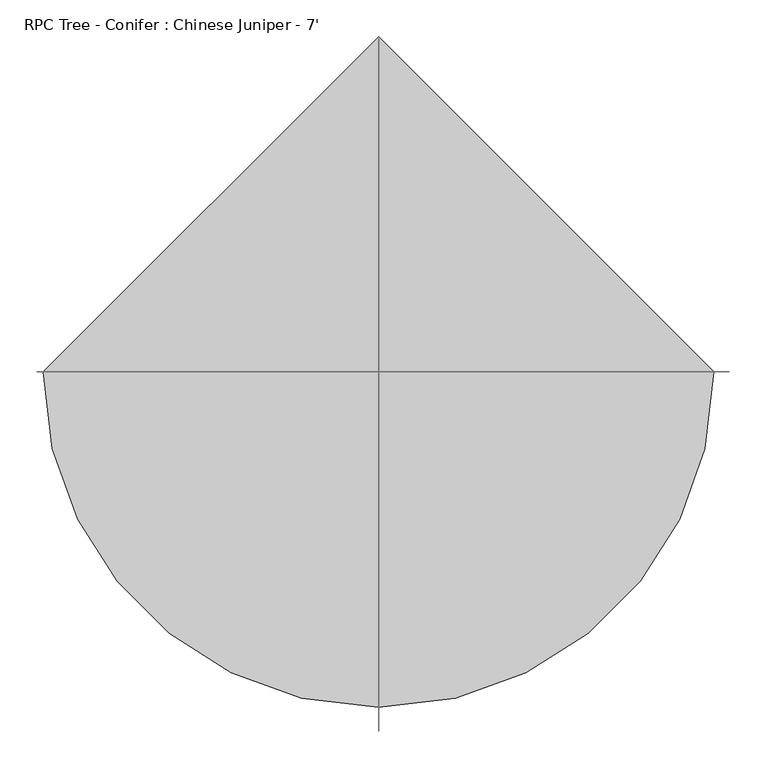
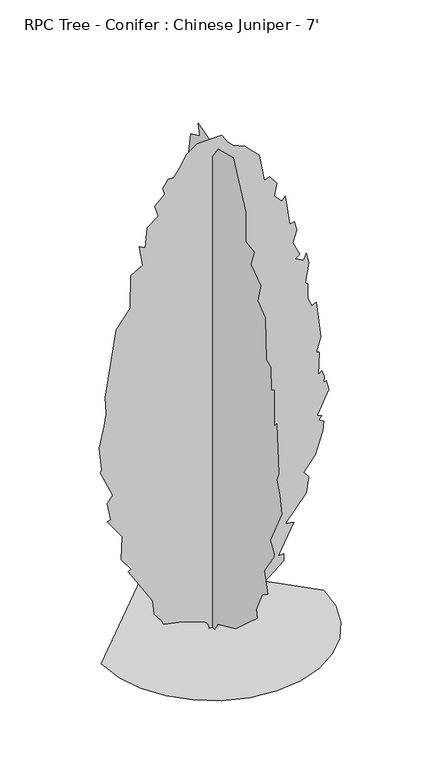
"""IFC4 building model written with IfcOpenShell, lengths in millimetres: geographic element geometry, RPC Tree - Conifer : Chinese Juniper - 7'."""

from ifc_helpers import new_model, si_unit, origin, place, context, project, spatial, triangles, source, transform, mapped, element, save


def rpc_tree_conifer_chinese_juniper_7_1b9786cd(model_context):
    return source(origin(), model_context, "Body", "Tessellation", [
        triangles([(-14.517647, 6e-07, 1.3e-06), (-18.0071097, -3e-07, 17.9396969), (-27.4223632, -6e-07, 30.3914521), (-123.5685295, 1.5e-06, 65.7757953), (-201.676062, 3.9e-06, 82.3498608), (-209.1624873, 3.1e-06, 101.0656516), (-239.326362, 2.1e-06, 139.6788561), (-246.5945957, -1e-06, 198.3880905), (-257.8249785, -1.9e-06, 220.8470939), (-347.6599566, -6.4e-06, 363.0865585), (-336.0369015, -7.4e-06, 370.071561), (-375.7854927, -8.9e-06, 425.7942498), (-371.7570322, -1.5e-05, 524.6285151), (-433.7535387, -1.74e-05, 610.1379032), (-418.7802157, -1.83e-05, 613.8793173), (-433.1718882, -2.22e-05, 689.5207758), (-411.2922644, -2.49e-05, 718.6876728), (-463.6977139, -2.95e-05, 834.7279736), (-456.2123059, -3.02e-05, 842.2133451), (-467.4416714, -3.58e-05, 943.2777431), (-447.126705, -4.19e-05, 1031.4541197), (-437.4949891, -4.53e-05, 1081.7767748), (-441.2389466, -4.94e-05, 1152.8969976), (-396.3214485, -6.81e-05, 1433.6338589), (-340.174585, -7.5e-05, 1508.4981846), (-337.1392688, -8.35e-05, 1648.2265743), (-287.7691355, -8.74e-05, 1676.941246), (-302.7424948, -9.18e-05, 1763.0323574), (-277.1874594, -9.21e-05, 1748.371479), (-269.0543621, -9.76e-05, 1834.1525803), (-224.1350836, -0.0001015, 1867.8406403), (-239.107916, -0.0001038, 1916.5022049), (-197.9328675, -0.0001078, 1953.9342224), (-205.4192747, -0.000109, 1980.1369835), (-182.9602713, -0.000112, 2013.8251888), (-160.5012679, -0.000113, 2013.8251888), (-134.7328734, -0.0001161, 2047.2821583), (-108.898967, -0.0001202, 2095.8470718), (-62.5486394, -0.0001241, 2127.2339642), (37.1144179, -0.0001285, 2128.801165), (60.3458442, -0.0001273, 2092.4307106), (82.8048476, -0.000127, 2069.9720524), (132.737601, -0.0001279, 2048.8239246), (191.3566519, -0.0001268, 1987.6224277), (213.8156735, -0.0001209, 1871.5845978), (236.2746769, -0.0001223, 1879.070042), (263.6666277, -0.0001212, 1839.8828991), (254.989959, -0.0001178, 1789.2351185), (284.9366594, -0.0001171, 1755.5469131), (299.9074571, -0.0001186, 1770.5202724), (318.6248102, -0.0001119, 1643.2505699), (337.3395836, -0.0001129, 1646.9946728), (347.517378, -0.0001111, 1609.9130699), (330.7888933, -0.0001074, 1559.0291119), (359.7983145, -0.000105, 1497.2687828), (340.1843954, -0.0001034, 1485.5084541), (374.7716738, -0.0001038, 1467.3220642), (386.0010392, -0.0001059, 1493.5248253), (397.230441, -0.0001037, 1448.6072182), (382.2596251, -9.81e-05, 1366.2577389), (393.0673594, -9.81e-05, 1357.3651131), (391.5662155, -9.44e-05, 1296.562429), (408.4598064, -9.28e-05, 1257.7053532), (427.1771233, -9.41e-05, 1265.1907974), (445.8918966, -8.55e-05, 1107.9794632), (427.1771233, -8.11e-05, 1048.0886421), (438.8332068, -8.14e-05, 1044.1287821), (434.6625312, -7.54e-05, 947.0217007), (449.6358905, -7.68e-05, 958.2511024), (460.8652559, -7.57e-05, 932.0483414), (457.1212984, -7.4e-05, 905.8481964), (468.3506639, -7.47e-05, 909.5896105), (479.5800293, -7.27e-05, 868.4161062), (430.9185737, -6.48e-05, 771.0931223), (449.6358905, -6.52e-05, 763.6077507), (438.4064887, -6.38e-05, 748.6343914), (457.1212984, -6.39e-05, 737.4049896), (453.1842567, -6.13e-05, 697.0620306), (423.4331657, -5.44e-05, 602.6499518), (374.7716738, -4.87e-05, 542.7590944), (397.230441, -4.81e-05, 516.5563697), (384.9545551, -4.37e-05, 451.166393), (299.9074571, -3.36e-05, 344.3717488), (333.5981332, -3.49e-05, 340.6277913), (269.9633001, -2.47e-05, 217.1038994), (292.4220673, -2.57e-05, 217.1038994), (292.4220673, -2.39e-05, 187.1584707), (127.7223548, -8.7e-06, 52.4044321), (127.7223548, -9.8e-06, 71.1202274), (15.4277284, -7e-07, 0.0), (0.1966721, 13.7891713, 0.00013), (0.1966737, 34.4811189, 14.2963339), (0.1966762, 77.4229995, 29.9456808), (0.1966783, 178.488651, 67.3772736), (0.1966827, 230.8930831, 116.0384931), (0.1966819, 208.4340797, 119.7817057), (0.1966904, 288.5449239, 235.2565704), (0.1966918, 264.5824875, 291.9663175), (0.196695, 331.9587347, 389.2892833), (0.1966967, 324.4733268, 434.2067814), (0.1967014, 373.1322753, 494.0976388), (0.1967052, 389.4924685, 565.7309481), (0.1967041, 380.6202267, 640.0820784), (0.1967106, 440.5110841, 729.9170746), (0.1967147, 444.2524981, 819.7546143), (0.196717, 422.6319428, 893.2725832), (0.1967196, 455.4818636, 1010.6565519), (0.19672, 425.5377248, 1051.8300562), (0.1967236, 388.1056346, 1171.611771), (0.1967244, 414.3083593, 1253.9613956), (0.1967283, 384.3616407, 1373.7430378), (0.1967298, 346.932094, 1444.8632607), (0.1967315, 328.2147772, 1594.5917667), (0.19673, 305.75601, 1583.362365), (0.1967359, 305.75601, 1718.1148956), (0.1967344, 260.8385118, 1729.3441521), (0.1967329, 237.0752094, 1809.303661), (0.1967352, 223.406676, 1875.3287006), (0.1967352, 178.488651, 1920.2461624), (0.1967401, 156.0296476, 2055.0011639), (0.1967346, 92.3955867, 2084.9454117), (0.1967371, 102.0598133, 2133.1292439), (0.1967319, 11.3487565, 2104.2112415), (0.1967329, 6.3027505, 2040.0278046), (0.1967297, -38.6152347, 2103.6627285), (0.1967262, -147.1670527, 2133.606831), (0.1967183, -237.0033388, 1950.1902649), (0.1967127, -237.0033388, 1822.9231785), (0.1967097, -296.2055936, 1812.3847229), (0.1967078, -270.691199, 1744.3175114), (0.1967065, -342.8426634, 1695.0642677), (0.196704, -323.0966666, 1617.050425), (0.1966999, -375.4995727, 1575.8744499), (0.1966957, -382.9874877, 1396.2018414), (0.1966938, -413.5488853, 1383.1639744), (0.1966894, -416.6756204, 1283.9081142), (0.196689, -439.1343876, 1298.8788574), (0.1966862, -439.1343876, 1141.6675959), (0.1966823, -457.849161, 1164.1263994), (0.1966765, -472.8225203, 954.5096884), (0.1966757, -456.5690065, 918.855542), (0.1966723, -480.3104716, 864.672076), (0.1966725, -491.5398371, 789.8078957), (0.1966689, -412.9316628, 628.8526766), (0.1966658, -439.1343876, 583.9351785), (0.1966692, -436.9195155, 568.0778978), (0.1966679, -368.0141647, 467.8974212), (0.1966629, -394.2168895, 381.8038754), (0.1966636, -353.0408054, 355.6011506), (0.1966655, -311.8672648, 265.7661362), (0.1966637, -319.3526728, 232.0767318), (0.196664, -244.4894916, 164.6997216), (0.1966643, -165.8828434, 93.5794897), (0.1966675, -34.8715179, 33.6886368), (0.1966708, -16.1562041, 0.0001282), (-457.9674314, 0.0, 0.0001492), (-445.8541446, -104.9808196, 0.0001424), (-411.358285, -201.3891246, 0.0001352), (-357.2408761, -286.4621113, 0.0001277), (-286.2654482, -357.4375574, 0.0001204), (-201.1924614, -411.5549664, 0.0001134), (-104.7841473, -446.0508259, 0.0001072), (0.1966917, -458.1641127, 0.0001019), (105.1774918, -446.0508259, 9.8e-05), (201.5857877, -411.5549664, 9.58e-05), (286.6587745, -357.4375574, 9.54e-05), (357.6342387, -286.4621113, 9.65e-05), (411.7516477, -201.3888702, 9.92e-05), (446.2475072, -104.9808196, 0.0001034), (458.360794, 4.01e-05, 0.0001092), (0.1966112, 458.1641127, 0.0001565)], [[57, 58, 59], [27, 28, 29], [87, 88, 89], [49, 50, 51], [13, 14, 15], [83, 84, 85], [74, 75, 76], [63, 64, 65], [68, 69, 70], [71, 72, 73], [9, 10, 11], [85, 86, 87], [85, 87, 89], [51, 52, 53], [54, 55, 56], [90, 1, 2], [66, 67, 68], [45, 46, 47], [17, 18, 19], [68, 70, 71], [45, 47, 48], [31, 32, 33], [76, 77, 78], [89, 90, 2], [89, 2, 3], [57, 59, 60], [51, 53, 54], [25, 26, 27], [39, 40, 41], [56, 57, 60], [71, 73, 74], [34, 35, 36], [33, 34, 36], [4, 5, 6], [60, 61, 62], [80, 81, 82], [38, 39, 41], [37, 38, 41], [37, 41, 42], [29, 30, 31], [15, 16, 17], [36, 37, 42], [33, 36, 42], [31, 33, 42], [31, 42, 43], [31, 43, 44], [31, 44, 45], [29, 31, 45], [29, 45, 48], [27, 29, 48], [25, 27, 48], [25, 48, 49], [25, 49, 51], [25, 51, 54], [25, 54, 56], [25, 56, 60], [25, 60, 62], [24, 25, 62], [23, 24, 62], [22, 23, 62], [22, 62, 63], [22, 63, 65], [22, 65, 66], [22, 66, 68], [21, 22, 68], [20, 21, 68], [19, 20, 68], [17, 19, 68], [17, 68, 71], [17, 71, 74], [15, 17, 74], [13, 15, 74], [13, 74, 76], [13, 76, 78], [13, 78, 79], [13, 79, 80], [12, 13, 80], [11, 12, 80], [9, 11, 80], [9, 80, 82], [9, 82, 83], [9, 83, 85], [9, 85, 89], [9, 89, 3], [9, 3, 4], [8, 9, 4], [8, 4, 6], [7, 8, 6], [138, 139, 140], [94, 95, 96], [136, 137, 138], [121, 122, 123], [112, 113, 114], [128, 129, 130], [121, 123, 124], [125, 126, 127], [124, 125, 127], [114, 115, 116], [147, 148, 149], [130, 131, 132], [124, 127, 128], [134, 135, 136], [154, 155, 91], [154, 91, 92], [150, 151, 152], [96, 97, 98], [119, 120, 121], [119, 121, 124], [119, 124, 128], [118, 119, 128], [117, 118, 128], [116, 117, 128], [116, 128, 130], [114, 116, 130], [114, 130, 132], [112, 114, 132], [112, 132, 133], [112, 133, 134], [112, 134, 136], [111, 112, 136], [110, 111, 136], [109, 110, 136], [109, 136, 138], [109, 138, 140], [109, 140, 141], [108, 109, 141], [107, 108, 141], [106, 107, 141], [105, 106, 141], [104, 105, 141], [103, 104, 141], [103, 141, 142], [103, 142, 143], [103, 143, 144], [102, 103, 144], [101, 102, 144], [100, 101, 144], [100, 144, 145], [100, 145, 146], [100, 146, 147], [100, 147, 149], [100, 149, 150], [100, 150, 152], [100, 152, 153], [100, 153, 154], [99, 100, 154], [98, 99, 154], [96, 98, 154], [96, 154, 92], [96, 92, 93], [96, 93, 94], [170, 171, 156], [169, 170, 156], [169, 156, 157], [168, 169, 157], [168, 157, 158], [168, 158, 159], [167, 168, 159], [166, 167, 159], [166, 159, 160], [166, 160, 161], [166, 161, 162], [166, 162, 163], [166, 163, 164], [166, 164, 165]], closed=False),
    ])


if __name__ == "__main__":
    model = new_model("IFC4")
    model_context = context("Model", 3, world=origin())
    ifc_project = project(units=[si_unit("LENGTHUNIT", "METRE", prefix="MILLI")], contexts=[model_context])
    site = spatial("IfcSite", under=ifc_project)
    building = spatial("IfcBuilding", under=site)
    placement = place(None, origin())
    rpc_tree_conifer_chinese_juniper_7_shape = rpc_tree_conifer_chinese_juniper_7_1b9786cd(model_context)
    element("IfcGeographicElement", 1, ObjectType="RPC Tree - Conifer : Chinese Juniper - 7'", at=placement, inside=building, context=model_context, shape_type="MappedRepresentation", body=[
        mapped(rpc_tree_conifer_chinese_juniper_7_shape, transform((0.0, 0.0, 0.0), x_axis=(1.0, 0.0, 0.0), y_axis=(0.0, 1.0, 0.0), z_axis=(0.0, 0.0, 1.0))),
    ])
    save(model, "model.ifc")

# Revit data of these elements
# Type "RPC Tree - Conifer : Chinese Juniper - 7'"
#   built-in parameter 1005198 = "{2, 15},{39, RPC-16-FUM3-UUQ0-UBF0-N000-ST1L-LVER-AU},{1, 0},{1, 0},{2, 35},{1, 8},{5, Color},{1, 0},{1, 0},{3, 0.8},{3, 0.8},{3, 0.8},{1, 8},{7, BBoxMin},{1, 0},{1, 0},{1, 0},{1, 0},{1, 0},{1, 8},{7, BBoxMax},{1, 0},{1, 0},{1, 0},{1, 0},{1, 0},{2, 11},{9, RPCTypeId},{1, 0},{1, 0},{39, RPC-16-FUM3-UUQ0-UBF0-N000-ST1L-LVER-AU},{1, 6},{14, RPCPlantHeight},{1, 0},{1, 0},{1, 7},{2, 11},{7, keyword},{1, 0},{1, 0},{96, :Geometry:RPC:Chinese Juniper:juniperus chinensis:chinese:juniper:cupressaceae:conifer:evergreen},{2, 11},{8, category},{1, 0},{1, 0},{16, :Trees [General]},{2, 11},{12, LocalizedUID},{1, 0},{1, 0},{15, Chinese Juniper},{2, 14},{6, Height},{1, 0},{1, 0},{1, 7},{1, 2},{16, Cast Reflections},{1, 0},{1, 0},{1, 0},{1, 2},{12, Cast Shadows},{1, 0},{1, 0},{1, 1},{1, 2},{9, Lock View},{1, 0},{1, 0},{1, 0},{1, 4},{5, ViewC},{1, 0},{1, 0},{1, 0},{2, 11},{20, AdvancedUIDefinition},{1, 0},{1, 0},{0, },{2, 11},{10, AssetLibID},{1, 0},{1, 0},{36, 4D3F6E72-3F99-4203-98E9-AF80B3C7A7A4},{2, 11},{10, BaseSchema},{1, 0},{1, 0},{9, RPCSchema},{2, 11},{12, ExchangeGUID},{1, 0},{1, 0},{0, },{1, 2},{6, Hidden},{1, 0},{1, 0},{1, 0},{1, 4},{11, RPCCategory},{1, 0},{1, 0},{1, 0},{2, 11},{8, RPCImage},{1, 0},{1, 0},{0, },{1, 4},{13, SchemaVersion},{1, 0},{1, 0},{1, 4},{2, 11},{12, UIDefinition},{1, 0},{1, 0},{0, },{2, 11},{6, UIName},{1, 0},{1, 0},{39, RPC-16-FUM3-UUQ0-UBF0-N000-ST1L-LVER-AU},{2, 11},{11, VersionGUID},{1, 0},{1, 0},{9, RPCSchema},{2, 11},{9, assettype},{1, 0},{1, 0},{11, RPCGeometry},{2, 11},{11, description},{1, 0},{1, 0},{0, },{2, 11},{9, localname},{1, 0},{1, 0},{3, RPC},{2, 11},{9, localtype},{1, 0},{1, 0},{3, RPC},{1, 4},{8, revision},{1, 0},{1, 0},{1, 1},{2, 11},{9, thumbnail},{1, 0},{1, 0},{0, },{1, 4},{7, version},{1, 0},{1, 0},{1, 1},{1, 2},{20, RPC_Cast Reflections},{1, 0},{1, 0},{1, 1},{1, 2},{16, RPC_Cast Shadows},{1, 0},{1, 0},{1, 1},{1, 2},{13, RPC_Lock View},{1, 0},{1, 0},{1, 0},{1, 4},{9, RPC_ViewC},{1, 0},{1, 0},{1, 0},{21, assetlibrary_base.fbx},{1, 5},"
#   built-in parameter 1005195 = "RPC-16-FUM3-UUQ0-UBF0-N000-ST1L-LVER-AU"
#   Type Comments = "Chinese Juniper"
#   Assembly Code = "G2050500"
#   Height = 7' - 0"
#   Description = (empty or 0)
#   Default Elevation = 0
